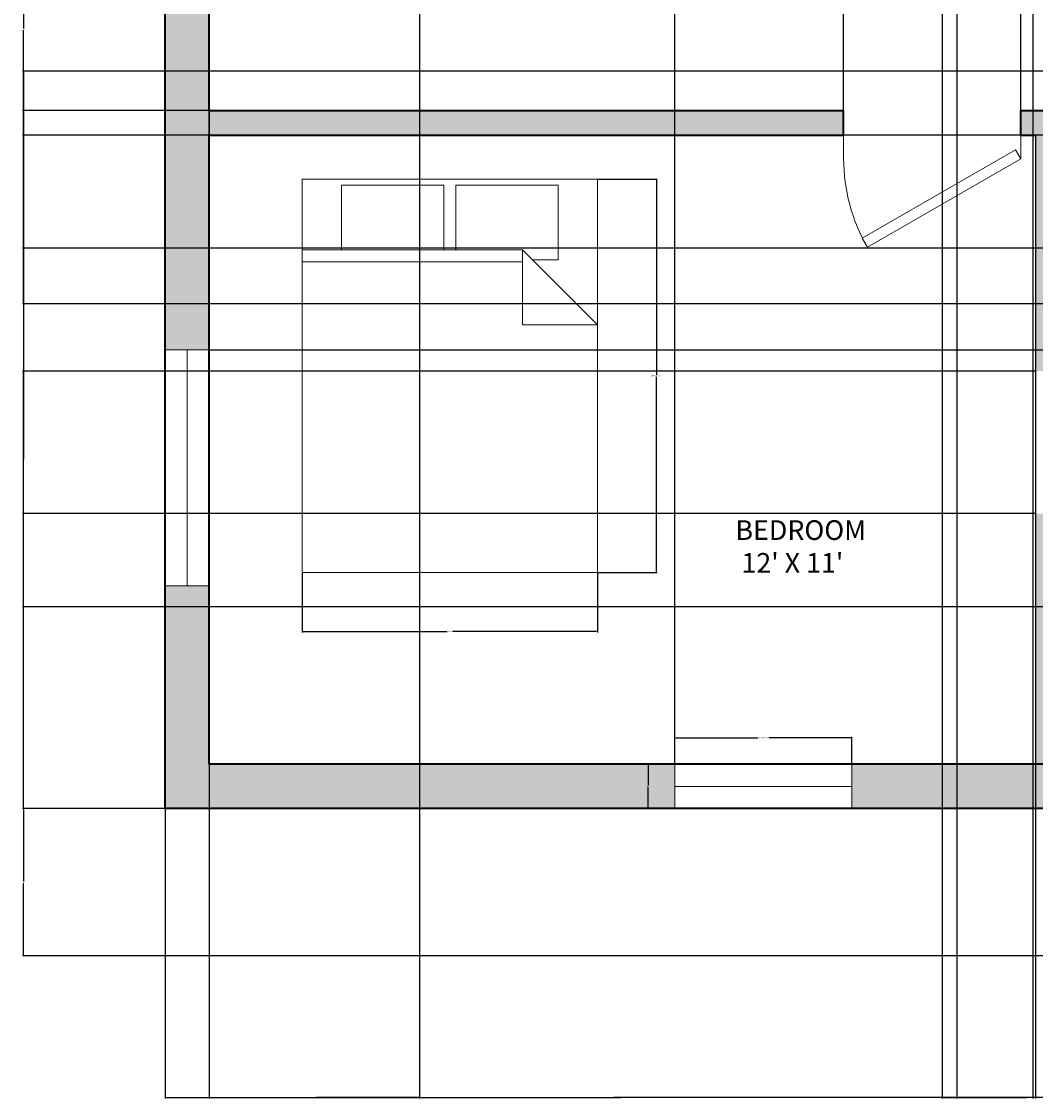
# Model space of a CAD drawing. Units: inches. Extents: x -28 to 649, y -11 to 509.
# Tile 1 of 7: x -2 to 204, y -11 to 208. Entities that reach past the tile are written whole.
import ezdxf

# ---------------------------------------------------------------- set-up
doc = ezdxf.new("R2010")
doc.units = ezdxf.units.IN
doc.header["$MEASUREMENT"] = 0
for name, color, linetype, lineweight in [('A-ANNO-DIMS', 2, 'Continuous', 18), ('A-AREA-IDEN', 18, 'Continuous', 18), ('A-WALL', 7, 'Continuous', 35), ('A-WALL-PATT', 251, 'Continuous', 13), ('doors', 40, 'Continuous', 20), ('furniture', 220, 'Continuous', 18), ('window', 30, 'Continuous', 18)]:
    doc.layers.add(name, color=color, linetype=linetype, lineweight=lineweight)
doc.styles.get("Standard").update_dxf_attribs({"font": 'arial.ttf'})
doc.dimstyles.get("Standard").update_dxf_attribs({"dimtxt": 0.18, "dimasz": 0.18, "dimexe": 0.18, "dimexo": 0.0625, "dimgap": 0.09, "dimtad": 0, "dimtih": 1, "dimtoh": 1, "dimdec": 4, "dimzin": 0, "dimdsep": 46, "dimtxsty": 'Standard', "dimcen": 0.09, "dimadec": 0, "dimazin": 0, "dimtfac": 1, "dimtdec": 4, "dimtofl": 0, "dimtmove": 0, "dimatfit": 3, "dimfxl": 1, "dimtolj": 1, "dimtzin": 0, "dimarcsym": 0})

# ---------------------------------------------------------------- blocks, each defined once
blk = doc.blocks.new('*U9')
for p, q in [((0, 0), (0, -100)), ((750, 0), (750, -100))]:
    blk.add_line(p, q)
blk.add_lwpolyline([(0, 0), (649.5, 375), (671.4, 337.1), (21.9, -37.9)], close=True)
blk.add_arc((0, 0), 750, 0, 30)
blk = doc.blocks.new('Bed - Queen')
for p, q in [((0, -80.00003), (0, 0)), ((0, 0), (59.99999, 0)), ((59.99999, 0), (59.99999, -80.00003)), ((7.99999, -1.2), (28.79998, -1.2)), ((7.99999, -14.4), (7.99999, -1.2)), ((28.79998, -1.2), (28.79998, -14.4)), ((31.19999, -1.2), (51.99999, -1.2)), ((31.19999, -14.4), (31.19999, -1.2)), ((51.99999, -1.2), (51.99999, -16.4)), ((0, -14.4), (44.8, -14.4)), ((59.99999, -29.6), (44.8, -14.4)), ((44.8, -14.4), (44.8, -29.6)), ((44.8, -16.8), (0, -16.8)), ((51.99999, -16.4), (46.79936, -16.4)), ((44.8, -29.6), (59.99999, -29.6)), ((59.99999, -80.00003), (0, -80.00003))]:
    blk.add_line(p, q)
blk = doc.blocks.new('WIN-48x9')
for p, q in [((9, 48), (0, 48)), ((0, 48), (0, 0)), ((4.5, 0), (4.5, 48)), ((9, 0), (9, 48)), ((0, 0), (9, 0)), ((0, 0), (4.5, 0))]:
    blk.add_line(p, q)
blk = doc.blocks.new('WIN-36x9')
for p, q in [((0, 9), (0, 0)), ((36, 9), (0, 9)), ((0, 9), (0, 4.5)), ((36, 0), (36, 9)), ((0, 4.5), (36, 4.5)), ((0, 0), (36, 0))]:
    blk.add_line(p, q)
blk = doc.blocks.new('*D16')
at = {"layer": 'A-ANNO-DIMS', "color": 0, "lineweight": -2, "transparency": 16777216}
for p, q in [((131.12, 57), (131.12, 62.52)), ((131.3, 62.34), (148, 62.34)), ((166.94, 62.34), (150.24, 62.34)), ((167.12, 57), (167.12, 62.52))]:
    blk.add_line(p, q, dxfattribs=at)
at = {"layer": 'A-ANNO-DIMS', "color": 0, "transparency": 16777216}
for points in [[(131.3, 62.37), (131.3, 62.31), (131.12, 62.34)], [(166.94, 62.37), (166.94, 62.31), (167.12, 62.34)]]:
    blk.add_solid(points, dxfattribs=at)
at = {"layer": 'Defpoints', "color": 0, "transparency": 16777216}
for p in [(167.12, 62.34), (131.12, 56.94), (167.12, 56.94)]:
    blk.add_point(p, dxfattribs=at)
at = {"layer": 'A-ANNO-DIMS', "color": 0, "transparency": 16777216, "insert": (149.12, 62.34), "char_height": 0.18, "attachment_point": 5}
blk.add_mtext('\\A1;WINDOW 36 TYP.', dxfattribs=at)
blk = doc.blocks.new('*D17')
at = {"layer": 'A-ANNO-DIMS', "color": 0, "lineweight": -2, "transparency": 16777216}
for p, q in [((131.06, 56.94), (125.54, 56.94)), ((125.72, 56.76), (125.72, 52.62)), ((125.72, 48.12), (125.72, 52.26)), ((131.06, 47.94), (125.54, 47.94))]:
    blk.add_line(p, q, dxfattribs=at)
at = {"layer": 'A-ANNO-DIMS', "color": 0, "transparency": 16777216}
for points in [[(125.69, 56.76), (125.75, 56.76), (125.72, 56.94)], [(125.69, 48.12), (125.75, 48.12), (125.72, 47.94)]]:
    blk.add_solid(points, dxfattribs=at)
at = {"layer": 'Defpoints', "color": 0, "transparency": 16777216}
for p in [(125.72, 56.94), (131.12, 56.94), (131.12, 47.94)]:
    blk.add_point(p, dxfattribs=at)
at = {"layer": 'A-ANNO-DIMS', "color": 0, "transparency": 16777216, "insert": (125.72, 52.44), "char_height": 0.18, "attachment_point": 5}
blk.add_mtext('\\A1;9 TYP.', dxfattribs=at)
blk = doc.blocks.new('*D20')
at = {"layer": 'A-ANNO-DIMS', "color": 0, "lineweight": -2, "transparency": 16777216}
for p, q in [((115.43, 175.96), (127.55, 175.96)), ((127.37, 175.78), (127.37, 136.15)), ((127.37, 96.14), (127.37, 135.78)), ((115.43, 95.96), (127.55, 95.96))]:
    blk.add_line(p, q, dxfattribs=at)
at = {"layer": 'A-ANNO-DIMS', "color": 0, "transparency": 16777216}
for points in [[(127.34, 175.78), (127.4, 175.78), (127.37, 175.96)], [(127.34, 96.14), (127.4, 96.14), (127.37, 95.96)]]:
    blk.add_solid(points, dxfattribs=at)
at = {"layer": 'Defpoints', "color": 0, "transparency": 16777216}
for p in [(115.37, 175.96), (127.37, 175.96), (115.37, 95.96)]:
    blk.add_point(p, dxfattribs=at)
at = {"layer": 'A-ANNO-DIMS', "color": 0, "transparency": 16777216, "insert": (127.37, 135.96), "char_height": 0.18, "attachment_point": 5}
blk.add_mtext('\\A1;QUEEN BED 80 TYP.', dxfattribs=at)
blk = doc.blocks.new('*D21')
at = {"layer": 'A-ANNO-DIMS', "color": 0, "lineweight": -2, "transparency": 16777216}
for p, q in [((55.37, 95.9), (55.37, 83.78)), ((115.37, 95.9), (115.37, 83.78)), ((55.55, 83.96), (84.84, 83.96)), ((115.19, 83.96), (85.9, 83.96))]:
    blk.add_line(p, q, dxfattribs=at)
at = {"layer": 'A-ANNO-DIMS', "color": 0, "transparency": 16777216}
for points in [[(55.55, 83.99), (55.55, 83.93), (55.37, 83.96)], [(115.19, 83.99), (115.19, 83.93), (115.37, 83.96)]]:
    blk.add_solid(points, dxfattribs=at)
at = {"layer": 'Defpoints', "color": 0, "transparency": 16777216}
for p in [(55.37, 95.96), (115.37, 95.96), (115.37, 83.96)]:
    blk.add_point(p, dxfattribs=at)
at = {"layer": 'A-ANNO-DIMS', "color": 0, "transparency": 16777216, "insert": (85.37, 83.96), "char_height": 0.18, "attachment_point": 5}
blk.add_mtext('\\A1;60 TYP.', dxfattribs=at)
blk = doc.blocks.new('*D32')
at = {"layer": 'A-ANNO-DIMS', "color": 0, "lineweight": -2, "transparency": 16777216}
for p, q in [((269.39, 47.94), (-1.53, 47.94)), ((-1.35, 47.76), (-1.35, 33.12)), ((-1.35, 18.12), (-1.35, 32.76)), ((269.39, 17.94), (-1.53, 17.94))]:
    blk.add_line(p, q, dxfattribs=at)
at = {"layer": 'A-ANNO-DIMS', "color": 0, "transparency": 16777216}
for points in [[(-1.38, 47.76), (-1.32, 47.76), (-1.35, 47.94)], [(-1.38, 18.12), (-1.32, 18.12), (-1.35, 17.94)]]:
    blk.add_solid(points, dxfattribs=at)
at = {"layer": 'Defpoints', "color": 0, "transparency": 16777216}
for p in [(269.45, 47.94), (-1.35, 17.94), (269.45, 17.94)]:
    blk.add_point(p, dxfattribs=at)
at = {"layer": 'A-ANNO-DIMS', "color": 0, "transparency": 16777216, "insert": (-1.35, 32.94), "char_height": 0.18, "attachment_point": 5}
blk.add_mtext('\\A1;30', dxfattribs=at)
blk = doc.blocks.new('*D35')
at = {"layer": 'A-ANNO-DIMS', "color": 0, "lineweight": -2, "transparency": 16777216}
for p, q in [((36.39, 189.94), (-1.53, 189.94)), ((-1.35, 189.76), (-1.35, 119.12)), ((-1.35, 48.12), (-1.35, 118.76)), ((27.39, 47.94), (-1.53, 47.94))]:
    blk.add_line(p, q, dxfattribs=at)
at = {"layer": 'A-ANNO-DIMS', "color": 0, "transparency": 16777216}
for points in [[(-1.38, 189.76), (-1.32, 189.76), (-1.35, 189.94)], [(-1.38, 48.12), (-1.32, 48.12), (-1.35, 47.94)]]:
    blk.add_solid(points, dxfattribs=at)
at = {"layer": 'Defpoints', "color": 0, "transparency": 16777216}
for p in [(-1.35, 189.94), (36.45, 189.94), (27.45, 47.94)]:
    blk.add_point(p, dxfattribs=at)
at = {"layer": 'A-ANNO-DIMS', "color": 0, "transparency": 16777216, "insert": (-1.35, 118.94), "char_height": 0.18, "attachment_point": 5}
blk.add_mtext('\\A1;142', dxfattribs=at)
blk = doc.blocks.new('*D37')
at = {"layer": 'A-ANNO-DIMS', "color": 0, "lineweight": -2, "transparency": 16777216}
for p, q in [((27.45, 47.88), (27.45, -11.04)), ((209.45, 47.88), (209.45, -11.04)), ((27.63, -10.86), (118.17, -10.86)), ((209.27, -10.86), (118.73, -10.86))]:
    blk.add_line(p, q, dxfattribs=at)
at = {"layer": 'A-ANNO-DIMS', "color": 0, "transparency": 16777216}
for points in [[(27.63, -10.83), (27.63, -10.89), (27.45, -10.86)], [(209.27, -10.83), (209.27, -10.89), (209.45, -10.86)]]:
    blk.add_solid(points, dxfattribs=at)
at = {"layer": 'Defpoints', "color": 0, "transparency": 16777216}
for p in [(27.45, 47.94), (209.45, 47.94), (209.45, -10.86)]:
    blk.add_point(p, dxfattribs=at)
at = {"layer": 'A-ANNO-DIMS', "color": 0, "transparency": 16777216, "insert": (118.45, -10.86), "char_height": 0.18, "attachment_point": 5}
blk.add_mtext('\\A1;182', dxfattribs=at)
blk = doc.blocks.new('*D44')
at = {"layer": 'A-ANNO-DIMS', "color": 0, "lineweight": -2, "transparency": 16777216}
for p, q in [((36.45, 470.88), (36.45, -11.04)), ((79.22, 470.88), (79.22, -11.04)), ((36.63, -10.86), (57.44, -10.86)), ((79.04, -10.86), (58.23, -10.86))]:
    blk.add_line(p, q, dxfattribs=at)
at = {"layer": 'A-ANNO-DIMS', "color": 0, "transparency": 16777216}
for points in [[(36.63, -10.83), (36.63, -10.89), (36.45, -10.86)], [(79.04, -10.83), (79.04, -10.89), (79.22, -10.86)]]:
    blk.add_solid(points, dxfattribs=at)
at = {"layer": 'Defpoints', "color": 0, "transparency": 16777216}
for p in [(36.45, 470.94), (79.22, 470.94), (79.22, -10.86)]:
    blk.add_point(p, dxfattribs=at)
at = {"layer": 'A-ANNO-DIMS', "color": 0, "transparency": 16777216, "insert": (57.83, -10.86), "char_height": 0.18, "attachment_point": 5}
blk.add_mtext('\\A1;42.77', dxfattribs=at)
blk = doc.blocks.new('*D45')
at = {"layer": 'A-ANNO-DIMS', "color": 0, "lineweight": -2, "transparency": 16777216}
for p, q in [((185.45, 470.88), (185.45, -11.04)), ((203.91, 470.88), (203.91, -11.04)), ((185.63, -10.86), (194.29, -10.86)), ((203.73, -10.86), (195.07, -10.86))]:
    blk.add_line(p, q, dxfattribs=at)
at = {"layer": 'A-ANNO-DIMS', "color": 0, "transparency": 16777216}
for points in [[(185.63, -10.83), (185.63, -10.89), (185.45, -10.86)], [(203.73, -10.83), (203.73, -10.89), (203.91, -10.86)]]:
    blk.add_solid(points, dxfattribs=at)
at = {"layer": 'Defpoints', "color": 0, "transparency": 16777216}
for p in [(185.45, 470.94), (203.91, 470.94), (203.91, -10.86)]:
    blk.add_point(p, dxfattribs=at)
at = {"layer": 'A-ANNO-DIMS', "color": 0, "transparency": 16777216, "insert": (194.68, -10.86), "char_height": 0.18, "attachment_point": 5}
blk.add_mtext('\\A1;18.46', dxfattribs=at)
blk = doc.blocks.new('*D52')
at = {"layer": 'A-ANNO-DIMS', "color": 0, "lineweight": -2, "transparency": 16777216}
for p, q in [((594.39, 262.25), (-1.53, 262.25)), ((-1.35, 262.07), (-1.35, 206.61)), ((-1.35, 150.79), (-1.35, 206.25)), ((594.39, 150.61), (-1.53, 150.61))]:
    blk.add_line(p, q, dxfattribs=at)
at = {"layer": 'A-ANNO-DIMS', "color": 0, "transparency": 16777216}
for points in [[(-1.38, 262.07), (-1.32, 262.07), (-1.35, 262.25)], [(-1.38, 150.79), (-1.32, 150.79), (-1.35, 150.61)]]:
    blk.add_solid(points, dxfattribs=at)
at = {"layer": 'Defpoints', "color": 0, "transparency": 16777216}
for p in [(-1.35, 262.25), (594.45, 262.25), (594.45, 150.61)]:
    blk.add_point(p, dxfattribs=at)
at = {"layer": 'A-ANNO-DIMS', "color": 0, "transparency": 16777216, "insert": (-1.35, 206.43), "char_height": 0.18, "attachment_point": 5}
blk.add_mtext('\\A1;111.64', dxfattribs=at)
blk = doc.blocks.new('*D53')
at = {"layer": 'A-ANNO-DIMS', "color": 0, "lineweight": -2, "transparency": 16777216}
for p, q in [((36.51, 241.9), (632.43, 241.9)), ((632.25, 241.72), (632.25, 191.76)), ((632.25, 141.44), (632.25, 191.39)), ((36.51, 141.26), (632.43, 141.26))]:
    blk.add_line(p, q, dxfattribs=at)
at = {"layer": 'A-ANNO-DIMS', "color": 0, "transparency": 16777216}
for points in [[(632.22, 241.72), (632.28, 241.72), (632.25, 241.9)], [(632.22, 141.44), (632.28, 141.44), (632.25, 141.26)]]:
    blk.add_solid(points, dxfattribs=at)
at = {"layer": 'Defpoints', "color": 0, "transparency": 16777216}
for p in [(36.45, 241.9), (632.25, 241.9), (36.45, 141.26)]:
    blk.add_point(p, dxfattribs=at)
at = {"layer": 'A-ANNO-DIMS', "color": 0, "transparency": 16777216, "insert": (632.25, 191.58), "char_height": 0.18, "attachment_point": 5}
blk.add_mtext('\\A1;100.64', dxfattribs=at)
blk = doc.blocks.new('*D55')
at = {"layer": 'A-ANNO-DIMS', "color": 0, "lineweight": -2, "transparency": 16777216}
for p, q in [((36.45, 57), (36.45, 508.92)), ((36.63, 508.74), (83.39, 508.74)), ((130.94, 508.74), (84.18, 508.74)), ((131.12, 57), (131.12, 508.92))]:
    blk.add_line(p, q, dxfattribs=at)
at = {"layer": 'A-ANNO-DIMS', "color": 0, "transparency": 16777216}
for points in [[(36.63, 508.77), (36.63, 508.71), (36.45, 508.74)], [(130.94, 508.77), (130.94, 508.71), (131.12, 508.74)]]:
    blk.add_solid(points, dxfattribs=at)
at = {"layer": 'Defpoints', "color": 0, "transparency": 16777216}
for p in [(131.12, 508.74), (36.45, 56.94), (131.12, 56.94)]:
    blk.add_point(p, dxfattribs=at)
at = {"layer": 'A-ANNO-DIMS', "color": 0, "transparency": 16777216, "insert": (83.79, 508.74), "char_height": 0.18, "attachment_point": 5}
blk.add_mtext('\\A1;94.67', dxfattribs=at)
blk = doc.blocks.new('*D57')
at = {"layer": 'A-ANNO-DIMS', "color": 0, "lineweight": -2, "transparency": 16777216}
for p, q in [((165.45, 190), (165.45, 508.92)), ((165.63, 508.74), (183.23, 508.74)), ((201.27, 508.74), (183.67, 508.74)), ((201.45, 190), (201.45, 508.92))]:
    blk.add_line(p, q, dxfattribs=at)
at = {"layer": 'A-ANNO-DIMS', "color": 0, "transparency": 16777216}
for points in [[(165.63, 508.77), (165.63, 508.71), (165.45, 508.74)], [(201.27, 508.77), (201.27, 508.71), (201.45, 508.74)]]:
    blk.add_solid(points, dxfattribs=at)
at = {"layer": 'Defpoints', "color": 0, "transparency": 16777216}
for p in [(201.45, 508.74), (165.45, 189.94), (201.45, 189.94)]:
    blk.add_point(p, dxfattribs=at)
at = {"layer": 'A-ANNO-DIMS', "color": 0, "transparency": 16777216, "insert": (183.45, 508.74), "char_height": 0.18, "attachment_point": 5}
blk.add_mtext('\\A1;36', dxfattribs=at)
blk = doc.blocks.new('*D58')
at = {"layer": 'A-ANNO-DIMS', "color": 0, "lineweight": -2, "transparency": 16777216}
for p, q in [((204.39, 136.94), (-1.53, 136.94)), ((-1.35, 136.76), (-1.35, 122.62)), ((-1.35, 108.12), (-1.35, 122.26)), ((204.39, 107.94), (-1.53, 107.94))]:
    blk.add_line(p, q, dxfattribs=at)
at = {"layer": 'A-ANNO-DIMS', "color": 0, "transparency": 16777216}
for points in [[(-1.38, 136.76), (-1.32, 136.76), (-1.35, 136.94)], [(-1.38, 108.12), (-1.32, 108.12), (-1.35, 107.94)]]:
    blk.add_solid(points, dxfattribs=at)
at = {"layer": 'Defpoints', "color": 0, "transparency": 16777216}
for p in [(-1.35, 136.94), (204.45, 136.94), (204.45, 107.94)]:
    blk.add_point(p, dxfattribs=at)
at = {"layer": 'A-ANNO-DIMS', "color": 0, "transparency": 16777216, "insert": (-1.35, 122.44), "char_height": 0.18, "attachment_point": 5}
blk.add_mtext('\\A1;29', dxfattribs=at)
blk = doc.blocks.new('*D59')
at = {"layer": 'A-ANNO-DIMS', "color": 0, "lineweight": -2, "transparency": 16777216}
for p, q in [((346.39, 197.94), (-1.53, 197.94)), ((-1.35, 197.76), (-1.35, 180.12)), ((-1.35, 162.12), (-1.35, 179.76)), ((346.39, 161.94), (-1.53, 161.94))]:
    blk.add_line(p, q, dxfattribs=at)
at = {"layer": 'A-ANNO-DIMS', "color": 0, "transparency": 16777216}
for points in [[(-1.38, 197.76), (-1.32, 197.76), (-1.35, 197.94)], [(-1.38, 162.12), (-1.32, 162.12), (-1.35, 161.94)]]:
    blk.add_solid(points, dxfattribs=at)
at = {"layer": 'Defpoints', "color": 0, "transparency": 16777216}
for p in [(-1.35, 197.94), (346.45, 197.94), (346.45, 161.94)]:
    blk.add_point(p, dxfattribs=at)
at = {"layer": 'A-ANNO-DIMS', "color": 0, "transparency": 16777216, "insert": (-1.35, 179.94), "char_height": 0.18, "attachment_point": 5}
blk.add_mtext('\\A1;36', dxfattribs=at)
blk = doc.blocks.new('*D62')
at = {"layer": 'A-ANNO-DIMS', "color": 0, "lineweight": -2, "transparency": 16777216}
for p, q in [((188.45, 381.88), (188.45, -11.04)), ((217.45, 381.88), (217.45, -11.04)), ((188.63, -10.86), (202.73, -10.86)), ((217.27, -10.86), (203.17, -10.86))]:
    blk.add_line(p, q, dxfattribs=at)
at = {"layer": 'A-ANNO-DIMS', "color": 0, "transparency": 16777216}
for points in [[(188.63, -10.83), (188.63, -10.89), (188.45, -10.86)], [(217.27, -10.83), (217.27, -10.89), (217.45, -10.86)]]:
    blk.add_solid(points, dxfattribs=at)
at = {"layer": 'Defpoints', "color": 0, "transparency": 16777216}
for p in [(188.45, 381.94), (217.45, 381.94), (217.45, -10.86)]:
    blk.add_point(p, dxfattribs=at)
at = {"layer": 'A-ANNO-DIMS', "color": 0, "transparency": 16777216, "insert": (202.95, -10.86), "char_height": 0.18, "attachment_point": 5}
blk.add_mtext('\\A1;29', dxfattribs=at)
blk = doc.blocks.new('*D72')
at = {"layer": 'A-ANNO-DIMS', "color": 0, "lineweight": -2, "transparency": 16777216}
for p, q in [((36.45, 184.88), (36.45, -11.04)), ((204.45, 184.88), (204.45, -11.04)), ((36.63, -10.86), (120.17, -10.86)), ((204.27, -10.86), (120.73, -10.86))]:
    blk.add_line(p, q, dxfattribs=at)
at = {"layer": 'A-ANNO-DIMS', "color": 0, "transparency": 16777216}
for points in [[(36.63, -10.83), (36.63, -10.89), (36.45, -10.86)], [(204.27, -10.83), (204.27, -10.89), (204.45, -10.86)]]:
    blk.add_solid(points, dxfattribs=at)
at = {"layer": 'Defpoints', "color": 0, "transparency": 16777216}
for p in [(36.45, 184.94), (204.45, 184.94), (204.45, -10.86)]:
    blk.add_point(p, dxfattribs=at)
at = {"layer": 'A-ANNO-DIMS', "color": 0, "transparency": 16777216, "insert": (120.45, -10.86), "char_height": 0.18, "attachment_point": 5}
blk.add_mtext('\\A1;168', dxfattribs=at)
blk = doc.blocks.new('*D73')
at = {"layer": 'A-ANNO-DIMS', "color": 0, "lineweight": -2, "transparency": 16777216}
for p, q in [((269.39, 184.94), (-1.53, 184.94)), ((-1.35, 184.76), (-1.35, 137.12)), ((-1.35, 89.12), (-1.35, 136.76)), ((269.39, 88.94), (-1.53, 88.94))]:
    blk.add_line(p, q, dxfattribs=at)
at = {"layer": 'A-ANNO-DIMS', "color": 0, "transparency": 16777216}
for points in [[(-1.38, 184.76), (-1.32, 184.76), (-1.35, 184.94)], [(-1.38, 89.12), (-1.32, 89.12), (-1.35, 88.94)]]:
    blk.add_solid(points, dxfattribs=at)
at = {"layer": 'Defpoints', "color": 0, "transparency": 16777216}
for p in [(-1.35, 184.94), (269.45, 184.94), (269.45, 88.94)]:
    blk.add_point(p, dxfattribs=at)
at = {"layer": 'A-ANNO-DIMS', "color": 0, "transparency": 16777216, "insert": (-1.35, 136.94), "char_height": 0.18, "attachment_point": 5}
blk.add_mtext('\\A1;96', dxfattribs=at)

msp = doc.modelspace()

# ---------------------------------------------------------------- hatches: boundary and pattern name
at = {"layer": 'A-WALL-PATT'}
h = msp.add_hatch(color=256, dxfattribs=at)
h.dxf.hatch_style = 1
h.paths.add_polyline_path([(36.4499, 184.9382), (165.4499, 184.9382), (165.4499, 189.9382), (36.4499, 189.9382), (36.4499, 241.898), (27.4499, 241.898), (27.4499, 141.2558), (36.4499, 141.2558)])
h.paths.add_polyline_path([(36.4499, 385.8835), (27.4499, 385.8835), (27.4499, 289.898), (36.4499, 289.898)])
h.paths.add_polyline_path([(185.4499, 341.9382), (180.4499, 341.9382), (180.4499, 338.9382), (36.4499, 338.9382), (36.4499, 333.9382), (185.4499, 333.9382)])
h.paths.add_polyline_path([(36.4499, 470.9382), (79.2168, 470.9382), (79.2168, 479.9382), (27.4499, 479.9382), (27.4499, 433.8835), (36.4499, 433.8835)])
h.paths.add_polyline_path([(185.4499, 470.9382), (203.9104, 470.9382), (203.9104, 479.9382), (127.2168, 479.9382), (127.2168, 470.9382), (180.4499, 470.9382), (180.4499, 381.9382), (188.4499, 381.9382), (188.4499, 386.9382), (185.4499, 386.9382)])
h.paths.add_polyline_path([(292.4601, 479.9382), (227.9104, 479.9382), (227.9104, 470.9382), (245.4499, 470.9382), (245.4499, 386.9382), (217.4499, 386.9382), (217.4499, 381.9382), (245.4499, 381.9382), (245.4499, 338.9382), (245.4499, 333.9382), (251.5222, 333.9382), (251.5222, 338.9382), (250.4499, 338.9382), (250.4499, 470.9382), (292.4601, 470.9382)])
h.paths.add_polyline_path([(410.9121, 479.9382), (340.4601, 479.9382), (340.4601, 470.9382), (382.4499, 470.9382), (382.4499, 338.9382), (287.5222, 338.9382), (287.5222, 333.9382), (387.4499, 333.9382), (387.4499, 381.9382), (415.4499, 381.9382), (415.4499, 386.9382), (387.4499, 386.9382), (387.4499, 470.9382), (410.9121, 470.9382)])
h.paths.add_polyline_path([(497.0961, 479.9382), (434.9121, 479.9382), (434.9121, 470.9382), (447.4499, 470.9382), (447.4499, 386.9382), (444.4499, 386.9382), (444.4499, 381.9382), (452.4499, 381.9382), (452.4499, 470.9382), (497.0961, 470.9382)])
h.paths.add_polyline_path([(603.4499, 479.9382), (545.0961, 479.9382), (545.0961, 470.9382), (594.4499, 470.9382), (594.4499, 418.4819), (603.4499, 418.4819)])
h.paths.add_polyline_path([(603.4499, 370.4819), (594.4499, 370.4819), (594.4499, 338.9382), (452.4499, 338.9382), (452.4499, 341.9382), (447.4499, 341.9382), (447.4499, 338.9382), (447.4499, 333.9382), (594.4499, 333.9382), (594.4499, 310.2528), (603.4499, 310.2528)])
h.paths.add_polyline_path([(603.4499, 262.2528), (594.4499, 262.2528), (594.4499, 205.9382), (515.4499, 205.9382), (515.4499, 200.9382), (594.4499, 200.9382), (594.4499, 150.6102), (603.4499, 150.6102)])
h = msp.add_hatch(color=256, dxfattribs=at)
h.dxf.hatch_style = 1
h.paths.add_polyline_path([(131.1226, 56.9382), (36.4499, 56.9382), (36.4499, 93.2558), (27.4499, 93.2558), (27.4499, 47.9382), (131.1226, 47.9382)])
h.paths.add_polyline_path([(204.4499, 56.9382), (167.1226, 56.9382), (167.1226, 47.9382), (204.4499, 47.9382)])
h.paths.add_polyline_path([(209.4499, 56.9382), (204.4499, 56.9382), (204.4499, 47.9382), (209.4499, 47.9382)])
h.paths.add_polyline_path([(209.4499, 83.9382), (237.8774, 83.9382), (237.8774, 88.9382), (209.4499, 88.9382), (209.4499, 107.9382), (204.4499, 107.9382), (204.4499, 56.9382), (209.4499, 56.9382)])
h.paths.add_polyline_path([(269.4499, 88.9382), (261.8774, 88.9382), (261.8774, 83.9382), (269.4499, 83.9382)], flags=17)
h.paths.add_polyline_path([(274.4499, 189.9382), (201.4499, 189.9382), (201.4499, 184.9382), (204.4499, 184.9382), (204.4499, 136.9382), (209.4499, 136.9382), (209.4499, 184.9382), (269.4499, 184.9382), (269.4499, 83.9382), (286.4499, 83.9382), (286.4499, 88.9382), (274.4499, 88.9382)])

# ---------------------------------------------------------------- linework, layer by layer
at = {"layer": 'A-WALL'}
for p, q in [((36.4499, 189.9382), (36.4499, 470.9382)), ((36.4499, 189.9382), (165.4499, 189.9382)), ((165.4499, 184.9382), (165.4499, 189.9382)), ((201.4499, 189.9382), (274.4499, 189.9382)), ((201.4499, 184.9382), (201.4499, 189.9382)), ((36.4499, 184.9382), (165.4499, 184.9382)), ((36.4499, 56.9382), (36.4499, 184.9382)), ((201.4499, 184.9382), (204.4499, 184.9382)), ((209.4499, 56.9382), (36.4499, 56.9382))]:
    msp.add_line(p, q, dxfattribs=at)
msp.add_lwpolyline([(209.4499, 47.9382), (27.4499, 47.9382), (27.4499, 479.9382), (603.4499, 479.9382), (603.4499, 47.9382), (269.4499, 47.9382)], dxfattribs=at)

# ---------------------------------------------------------------- block references
at = {"layer": 'doors', "xscale": 0.0479999999999998, "yscale": 0.0479999999999998, "zscale": 0.0479999999999998, "rotation": 180}
msp.add_blockref('*U9', (201.4499, 180.1382), dxfattribs=at)
at = {"layer": 'furniture'}
msp.add_blockref('Bed - Queen', (55.368, 175.9641), dxfattribs=at)
at = {"layer": 'window'}
for name, p in [('WIN-48x9', (27.4499, 93.2558)), ('WIN-36x9', (131.1226, 47.9382))]:
    msp.add_blockref(name, p, dxfattribs=at)

# ---------------------------------------------------------------- texts
at = {"layer": 'A-AREA-IDEN', "insert": (143.4419, 106.5785), "char_height": 4, "attachment_point": 1}
msp.add_mtext_dynamic_manual_height_columns("BEDROOM\\P 12' X 11'", width=46.696275, gutter_width=1, heights=[0], dxfattribs=at)

# ---------------------------------------------------------------- dimensions: what is measured, and where the dimension line sits
at = {"layer": 'A-ANNO-DIMS'}
for base, p1, p2, override, picture, middle in [((131.1226, 508.7392), (36.4499, 56.9382), (131.1226, 56.9382), {"dimdec": 2, "dimlfac": 1, "dimrnd": 0, "dimzin": 0, "dimdsep": 46, "dimlunit": 2}, '*D55', (83.7862, 508.7392)), ((201.4499, 508.7392), (165.4499, 189.9382), (201.4499, 189.9382), {"dimdec": 0, "dimlfac": 1, "dimrnd": 0, "dimzin": 0, "dimdsep": 46, "dimlunit": 2}, '*D57', (183.4499, 508.7392)), ((79.2168, -10.8628), (36.4499, 470.9382), (79.2168, 470.9382), {"dimdec": 2, "dimlfac": 1, "dimrnd": 0, "dimzin": 0, "dimdsep": 46, "dimlunit": 2}, '*D44', (57.8333, -10.8628)), ((203.9104, -10.8628), (185.4499, 470.9382), (203.9104, 470.9382), {"dimdec": 2, "dimlfac": 1, "dimrnd": 0, "dimzin": 0, "dimdsep": 46, "dimlunit": 2}, '*D45', (194.6801, -10.8628)), ((217.4499, -10.8628), (188.4499, 381.9382), (217.4499, 381.9382), {"dimdec": 0, "dimlfac": 1, "dimrnd": 0, "dimzin": 0, "dimdsep": 46, "dimlunit": 2}, '*D62', (202.9499, -10.8628)), ((204.4499, -10.8628), (36.4499, 184.9382), (204.4499, 184.9382), {"dimdec": 0, "dimlfac": 1, "dimrnd": 0, "dimzin": 0, "dimdsep": 46, "dimlunit": 2}, '*D72', (120.4499, -10.8628)), ((209.4499, -10.8628), (27.4499, 47.9382), (209.4499, 47.9382), {"dimdec": 0, "dimlfac": 1, "dimrnd": 0, "dimzin": 0, "dimdsep": 46, "dimlunit": 2}, '*D37', (118.4499, -10.8628))]:
    dim = msp.add_linear_dim(base=base, p1=p1, p2=p2, dimstyle='Standard', override=override, dxfattribs=at)
    dim.commit()
    dim.dimension.update_dxf_attribs({"geometry": picture, "text_midpoint": middle})
for base, p1, p2, override, picture, middle in [((-1.3511, 262.2528), (594.4499, 150.6102), (594.4499, 262.2528), {"dimdec": 2, "dimlfac": 1, "dimrnd": 0, "dimzin": 0, "dimdsep": 46, "dimlunit": 2}, '*D52', (-1.3511, 206.4315)), ((632.2509, 241.898), (36.4499, 141.2558), (36.4499, 241.898), {"dimdec": 2, "dimlfac": 1, "dimrnd": 0, "dimzin": 0, "dimdsep": 46, "dimlunit": 2}, '*D53', (632.2509, 191.5769)), ((-1.3511, 197.9382), (346.4499, 161.9382), (346.4499, 197.9382), {"dimdec": 0, "dimlfac": 1, "dimrnd": 0, "dimzin": 0, "dimdsep": 46, "dimlunit": 2}, '*D59', (-1.3511, 179.9382)), ((-1.3511, 189.9382), (27.4499, 47.9382), (36.4499, 189.9382), {"dimdec": 0, "dimlfac": 1, "dimrnd": 0, "dimzin": 0, "dimdsep": 46, "dimlunit": 2}, '*D35', (-1.3511, 118.9382)), ((-1.3511, 184.9382), (269.4499, 88.9382), (269.4499, 184.9382), {"dimdec": 0, "dimlfac": 1, "dimrnd": 0, "dimzin": 0, "dimdsep": 46, "dimlunit": 2}, '*D73', (-1.3511, 136.9382)), ((-1.3511, 136.9382), (204.4499, 107.9382), (204.4499, 136.9382), {"dimdec": 0, "dimlfac": 1, "dimrnd": 0, "dimzin": 0, "dimdsep": 46, "dimlunit": 2}, '*D58', (-1.3511, 122.4382)), ((-1.3511, 17.9382), (269.4499, 47.9382), (269.4499, 17.9382), {"dimdec": 0, "dimlfac": 1, "dimrnd": 0, "dimzin": 0, "dimdsep": 46, "dimlunit": 2}, '*D32', (-1.3511, 32.9382))]:
    dim = msp.add_linear_dim(base=base, p1=p1, p2=p2, angle=90, dimstyle='Standard', override=override, dxfattribs=at)
    dim.commit()
    dim.dimension.update_dxf_attribs({"geometry": picture, "text_midpoint": middle})
for base, p1, p2, text, picture, middle in [((127.368, 175.9641), (115.368, 95.964), (115.368, 175.9641), 'QUEEN BED <> TYP.', '*D20', (127.368, 135.964)), ((125.7226, 56.9382), (131.1226, 47.9382), (131.1226, 56.9382), '<> TYP.', '*D17', (125.7226, 52.4382))]:
    dim = msp.add_linear_dim(base=base, p1=p1, p2=p2, angle=90, text=text, dimstyle='Standard', override={"dimdec": 0, "dimlfac": 1, "dimrnd": 0, "dimzin": 0, "dimdsep": 46, "dimlunit": 2}, dxfattribs=at)
    dim.commit()
    dim.dimension.update_dxf_attribs({"geometry": picture, "text_midpoint": middle})
for base, p1, p2, text, picture, middle in [((115.368, 83.964), (55.368, 95.964), (115.368, 95.964), '<> TYP.', '*D21', (85.368, 83.964)), ((167.1226, 62.3382), (131.1226, 56.9382), (167.1226, 56.9382), 'WINDOW <> TYP.', '*D16', (149.1226, 62.3382))]:
    dim = msp.add_linear_dim(base=base, p1=p1, p2=p2, text=text, dimstyle='Standard', override={"dimdec": 0, "dimlfac": 1, "dimrnd": 0, "dimzin": 0, "dimdsep": 46, "dimlunit": 2}, dxfattribs=at)
    dim.commit()
    dim.dimension.update_dxf_attribs({"geometry": picture, "text_midpoint": middle})

doc.saveas('drawing.dxf')
